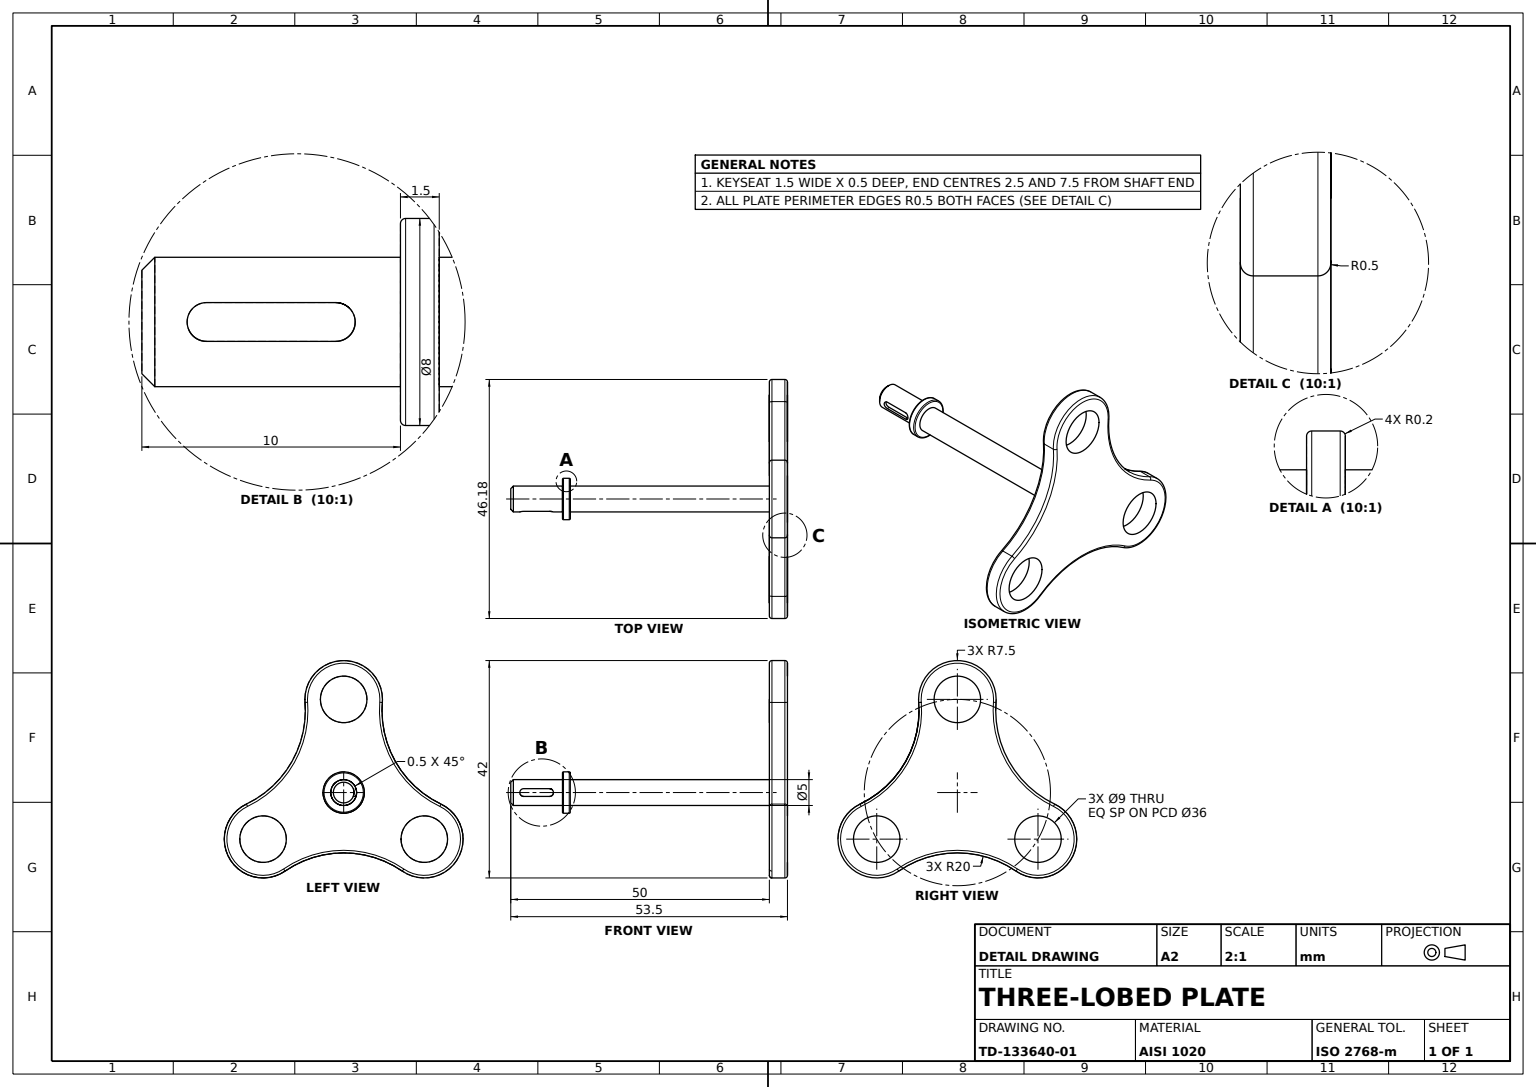
from build123d import *

# Parameters (mm, degrees)
CARRIER_PLATE_PROFILE_R   = 7.5
CARRIER_PLATE_PROFILE_R_2 = 4.5
CARRIER_PLATE_DEPTH       = 3.5
SHAFT_PROFILE_5_R         = 2.5
SHAFT_5X50_DEPTH          = 50
SHAFT_START               = -10
COLLAR_PROFILE_R          = 4
SHAFT_COLLAR_DEPTH        = 1.5
SHAFT_KEYSEAT_REACH       = 70.605
SHAFT_KEYSEAT_END_RADIUS  = 2
SHAFT_START_2             = 5
SHAFT_END_CHAMFER_SIZE    = 0.5
COLLAR_EDGE_FILLET_R      = 0.2
PLATE_EDGE_FILLET_R       = 0.5


with BuildPart() as part:
    # Carrier Plate Profile → Carrier Plate (new body)
    # profile 1 of 4: a face of its own
    with BuildSketch(Plane.XY):
        with Locations((15.588457268, -9)):
            Circle(CARRIER_PLATE_PROFILE_R)
        with Locations((15.588457268, -9)):
            Circle(CARRIER_PLATE_PROFILE_R_2, mode=Mode.SUBTRACT)
    # profile 2 of 4: a face of its own
    with BuildSketch(Plane.XY):
        with Locations((0, 18)):
            Circle(CARRIER_PLATE_PROFILE_R)
        with Locations((0, 18)):
            Circle(CARRIER_PLATE_PROFILE_R_2, mode=Mode.SUBTRACT)
    # profile 3 of 4: a face of its own
    with BuildSketch(Plane.XY):
        with Locations((-15.588457268, -9)):
            Circle(CARRIER_PLATE_PROFILE_R)
        with Locations((-15.588457268, -9)):
            Circle(CARRIER_PLATE_PROFILE_R_2, mode=Mode.SUBTRACT)
    # profile 4 of 4: a face of its own
    with BuildSketch(Plane.XY):
        with BuildLine():
            ThreePointArc((7.476559852, 17.407502934), (0, 10.5), (-7.476559852, 17.407502934))
            ThreePointArc((-7.476559852, 17.407502934), (-10.093544717, 5.827510759), (-18.813619684, -2.228860702))
            ThreePointArc((-18.813619684, -2.228860702), (-11.584628982, -2.658126534), (-8.088457268, -9))
            ThreePointArc((-8.088457268, -9), (-8.950103527, -12.490309386), (-11.337059831, -15.178642232))
            ThreePointArc((-11.337059831, -15.178642232), (0, -11.655021518), (11.337059831, -15.178642232))
            ThreePointArc((11.337059831, -15.178642232), (9.09326674, -5.25), (18.813619684, -2.228860702))
            ThreePointArc((18.813619684, -2.228860702), (10.093544717, 5.827510759), (7.476559852, 17.407502934))
        make_face()
    extrude(amount=CARRIER_PLATE_DEPTH)

    # Shaft Profile Ø5 → Shaft Ø5x50 (add)
    with BuildSketch(Plane.XY.offset(3.5)):
        Circle(SHAFT_PROFILE_5_R)
    extrude(amount=SHAFT_5X50_DEPTH)

    # Collar Profile → Shaft Collar (add)
    with BuildSketch(Plane.XY.offset(53.5).offset(SHAFT_START)):
        Circle(COLLAR_PROFILE_R)
    extrude(amount=-SHAFT_COLLAR_DEPTH)

    # Shaft Keyseat: up to this cylinder (the profile starts outside it)
    shaft_keyseat_end = Plane(origin=(0, 0, 48.5), z_dir=(0, 0, -1)) * Cylinder(SHAFT_KEYSEAT_END_RADIUS, 146.21, mode=Mode.PRIVATE)
    # Keyseat Profile → Shaft Keyseat (cut, up to the surface)
    with BuildSketch(Plane(origin=(0, 0, 0), x_dir=(0, 0, -1), z_dir=(1, 0, 0)).offset(SHAFT_START_2), mode=Mode.PRIVATE) as shaft_keyseat_sk1:
        with BuildLine():
            Line((-51, 0.75), (-46, 0.75))
            ThreePointArc((-46, 0.75), (-45.25, 0), (-46, -0.75))
            Line((-46, -0.75), (-51, -0.75))
            ThreePointArc((-51, -0.75), (-51.75, 0), (-51, 0.75))
        make_face()
    shaft_keyseat_tool1 = extrude(shaft_keyseat_sk1.sketch, amount=-SHAFT_KEYSEAT_REACH, mode=Mode.PRIVATE) - shaft_keyseat_end
    add(shaft_keyseat_tool1.solids().sort_by_distance((5, 0, 48.5))[0], mode=Mode.SUBTRACT)

    # Shaft End Chamfer
    shaft_end_chamfer_edges = [part.edges().sort_by_distance(p)[0] for p in [
        (-2.5, 0, 53.5),
    ]]
    chamfer(shaft_end_chamfer_edges, length=SHAFT_END_CHAMFER_SIZE)

    # Collar Edge Fillet
    collar_edge_fillet_edges = [part.edges().sort_by_distance(p)[0] for p in [
        (-4, 0, 42),
        (-4, 0, 43.5),
    ]]
    fillet(collar_edge_fillet_edges, radius=COLLAR_EDGE_FILLET_R)

    # Plate Edge Fillet
    plate_edge_fillet_edges = [part.edges().sort_by_distance(p)[0] for p in [
        (0, -11.655021518, 0),
        (-22.083647797, -12.75, 0),
        (22.083647797, -12.75, 3.5),
        (-10.093544717, 5.827510759, 0),
        (0, 25.5, 0),
        (10.093544717, 5.827510759, 0),
        (22.083647797, -12.75, 0),
        (10.093544717, 5.827510759, 3.5),
        (0, 25.5, 3.5),
        (-10.093544717, 5.827510759, 3.5),
        (-22.083647797, -12.75, 3.5),
        (0, -11.655021518, 3.5),
    ]]
    fillet(plate_edge_fillet_edges, radius=PLATE_EDGE_FILLET_R)


solid = part.part
